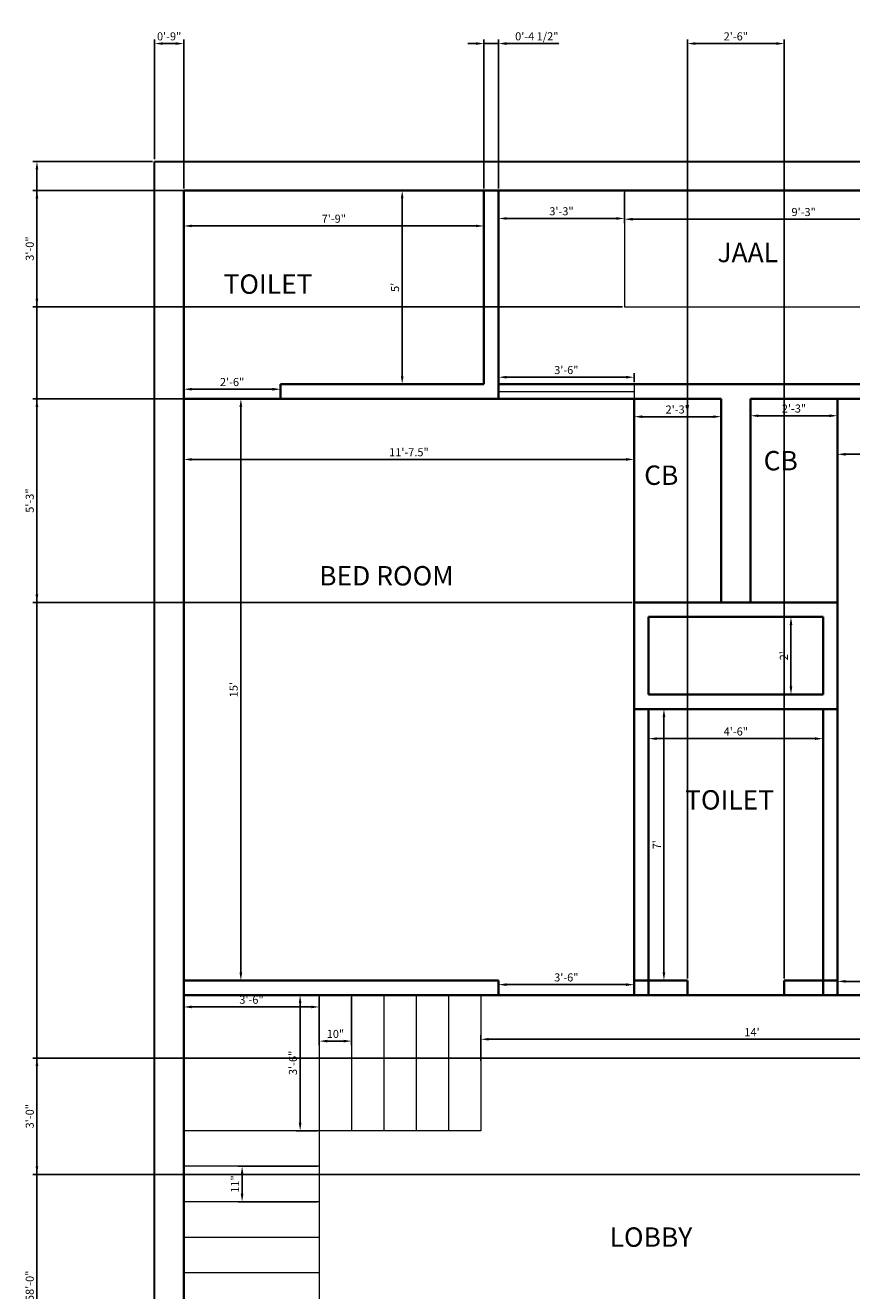
# Model space of a CAD drawing. Units: inches. Extents: x 2279 to 2719, y 394 to 1171.
# Tile 2 of 3: x 2281 to 2537, y 779 to 1171. Entities that reach past the tile are written whole.
import ezdxf

# ---------------------------------------------------------------- set-up
doc = ezdxf.new("R2010")
doc.units = ezdxf.units.IN
for name, color, linetype, lineweight in [('A-ANNO-DIMS', 2, 'Continuous', 13), ('A-ANNO-TEXT', 7, 'Continuous', 18), ('A-AREA-IDEN', 7, 'Continuous', 25), ('A-FLOR-OPEN', 4, 'Continuous', 18), ('A-FLOR-STRS', 3, 'Continuous', 20), ('A-GLAZ', 4, 'Continuous', 18), ('A-WALL', 7, 'Continuous', 35), ('C-PROP', 7, 'Continuous', 30)]:
    doc.layers.add(name, color=color, linetype=linetype, lineweight=lineweight)
doc.styles.get("Standard").update_dxf_attribs({"font": 'arial.ttf'})
doc.dimstyles.new('ISO-25', dxfattribs={"dimtxt": 2.5, "dimasz": 2.5, "dimexe": 1.25, "dimexo": 0.625, "dimtad": 1, "dimdec": 1, "dimlunit": 3, "dimtxsty": 'Standard', "dimcen": 2.5, "dimadec": 0, "dimazin": 0, "dimtfac": 1, "dimtdec": 1, "dimtmove": 0, "dimatfit": 3, "dimfxl": 1, "dimarcsym": 0})

# ---------------------------------------------------------------- blocks, each defined once
blk = doc.blocks.new('*D1')
at = {"layer": 'A-ANNO-DIMS', "color": 0, "lineweight": -2, "transparency": 16777216}
for p, q in [((2330.14, 1118.83), (2330.14, 1107.21)), ((2423.14, 1118.83), (2423.14, 1107.21)), ((2332.64, 1108.46), (2420.64, 1108.46))]:
    blk.add_line(p, q, dxfattribs=at)
at = {"layer": 'A-ANNO-DIMS', "color": 0, "transparency": 16777216}
for points in [[(2332.64, 1108.88), (2332.64, 1108.05), (2330.14, 1108.46)], [(2420.64, 1108.88), (2420.64, 1108.05), (2423.14, 1108.46)]]:
    blk.add_solid(points, dxfattribs=at)
at = {"layer": 'Defpoints', "color": 0, "transparency": 16777216}
for p in [(2330.14, 1119.45), (2423.14, 1119.45), (2423.14, 1108.46)]:
    blk.add_point(p, dxfattribs=at)
at = {"layer": 'A-ANNO-DIMS', "color": 0, "transparency": 16777216, "insert": (2376.64, 1110.37), "char_height": 2.5, "attachment_point": 5}
blk.add_mtext('7\'-9"', dxfattribs=at)
blk = doc.blocks.new('*D2')
at = {"layer": 'A-ANNO-DIMS', "color": 0, "lineweight": -2, "transparency": 16777216}
for p, q in [((2422.52, 1119.45), (2396.56, 1119.45)), ((2397.81, 1116.95), (2397.81, 1061.95)), ((2422.52, 1059.45), (2396.56, 1059.45))]:
    blk.add_line(p, q, dxfattribs=at)
at = {"layer": 'A-ANNO-DIMS', "color": 0, "transparency": 16777216}
for points in [[(2397.4, 1116.95), (2398.23, 1116.95), (2397.81, 1119.45)], [(2397.4, 1061.95), (2398.23, 1061.95), (2397.81, 1059.45)]]:
    blk.add_solid(points, dxfattribs=at)
at = {"layer": 'Defpoints', "color": 0, "transparency": 16777216}
for p in [(2423.14, 1119.45), (2397.81, 1059.45), (2423.14, 1059.45)]:
    blk.add_point(p, dxfattribs=at)
at = {"layer": 'A-ANNO-DIMS', "color": 0, "transparency": 16777216, "insert": (2395.92, 1089.45), "char_height": 2.5, "attachment_point": 5, "rotation": 90}
blk.add_mtext("5'", dxfattribs=at)
blk = doc.blocks.new('*D3')
at = {"layer": 'A-ANNO-DIMS', "color": 0, "lineweight": -2, "transparency": 16777216}
for p, q in [((2427.64, 1118.83), (2427.64, 1109.52)), ((2466.64, 1118.83), (2466.64, 1109.52)), ((2430.14, 1110.77), (2464.14, 1110.77))]:
    blk.add_line(p, q, dxfattribs=at)
at = {"layer": 'A-ANNO-DIMS', "color": 0, "transparency": 16777216}
for points in [[(2430.14, 1111.19), (2430.14, 1110.35), (2427.64, 1110.77)], [(2464.14, 1111.19), (2464.14, 1110.35), (2466.64, 1110.77)]]:
    blk.add_solid(points, dxfattribs=at)
at = {"layer": 'Defpoints', "color": 0, "transparency": 16777216}
for p in [(2427.64, 1119.45), (2466.64, 1119.45), (2466.64, 1110.77)]:
    blk.add_point(p, dxfattribs=at)
at = {"layer": 'A-ANNO-DIMS', "color": 0, "transparency": 16777216, "insert": (2447.14, 1112.67), "char_height": 2.5, "attachment_point": 5}
blk.add_mtext('3\'-3"', dxfattribs=at)
blk = doc.blocks.new('*D5')
at = {"layer": 'A-ANNO-DIMS', "color": 0, "lineweight": -2, "transparency": 16777216}
for p, q in [((2466.64, 1118.83), (2466.64, 1109.29)), ((2577.64, 1118.83), (2577.64, 1109.29)), ((2469.14, 1110.54), (2575.14, 1110.54))]:
    blk.add_line(p, q, dxfattribs=at)
at = {"layer": 'A-ANNO-DIMS', "color": 0, "transparency": 16777216}
for points in [[(2469.14, 1110.95), (2469.14, 1110.12), (2466.64, 1110.54)], [(2575.14, 1110.95), (2575.14, 1110.12), (2577.64, 1110.54)]]:
    blk.add_solid(points, dxfattribs=at)
at = {"layer": 'Defpoints', "color": 0, "transparency": 16777216}
for p in [(2466.64, 1119.45), (2577.64, 1119.45), (2577.64, 1110.54)]:
    blk.add_point(p, dxfattribs=at)
at = {"layer": 'A-ANNO-DIMS', "color": 0, "transparency": 16777216, "insert": (2522.14, 1112.44), "char_height": 2.5, "attachment_point": 5}
blk.add_mtext('9\'-3"', dxfattribs=at)
blk = doc.blocks.new('*D9')
at = {"layer": 'A-ANNO-DIMS', "color": 0, "lineweight": -2, "transparency": 16777216}
for p, q in [((2330.14, 1054.33), (2330.14, 1034.95)), ((2469.64, 1054.33), (2469.64, 1034.95)), ((2332.64, 1036.2), (2467.14, 1036.2))]:
    blk.add_line(p, q, dxfattribs=at)
at = {"layer": 'A-ANNO-DIMS', "color": 0, "transparency": 16777216}
for points in [[(2332.64, 1036.62), (2332.64, 1035.78), (2330.14, 1036.2)], [(2467.14, 1036.62), (2467.14, 1035.78), (2469.64, 1036.2)]]:
    blk.add_solid(points, dxfattribs=at)
at = {"layer": 'Defpoints', "color": 0, "transparency": 16777216}
for p in [(2330.14, 1054.95), (2469.64, 1054.95), (2469.64, 1036.2)]:
    blk.add_point(p, dxfattribs=at)
at = {"layer": 'A-ANNO-DIMS', "color": 0, "transparency": 16777216, "insert": (2399.89, 1038.1), "char_height": 2.5, "attachment_point": 5}
blk.add_mtext('11\'-7.5"', dxfattribs=at)
blk = doc.blocks.new('*D10')
at = {"layer": 'A-ANNO-DIMS', "color": 0, "lineweight": -2, "transparency": 16777216}
for p, q in [((2330.77, 1054.95), (2349.09, 1054.95)), ((2347.84, 1052.45), (2347.84, 877.45)), ((2330.77, 874.95), (2349.09, 874.95))]:
    blk.add_line(p, q, dxfattribs=at)
at = {"layer": 'A-ANNO-DIMS', "color": 0, "transparency": 16777216}
for points in [[(2347.42, 1052.45), (2348.26, 1052.45), (2347.84, 1054.95)], [(2347.42, 877.45), (2348.26, 877.45), (2347.84, 874.95)]]:
    blk.add_solid(points, dxfattribs=at)
at = {"layer": 'Defpoints', "color": 0, "transparency": 16777216}
for p in [(2330.14, 1054.95), (2330.14, 874.95), (2347.84, 874.95)]:
    blk.add_point(p, dxfattribs=at)
at = {"layer": 'A-ANNO-DIMS', "color": 0, "transparency": 16777216, "insert": (2345.94, 964.95), "char_height": 2.5, "attachment_point": 5, "rotation": 90}
blk.add_mtext("15'", dxfattribs=at)
blk = doc.blocks.new('*D11')
at = {"layer": 'A-ANNO-DIMS', "color": 0, "lineweight": -2, "transparency": 16777216}
for p, q in [((2469.64, 1054.33), (2469.64, 1048.18)), ((2496.64, 1054.33), (2496.64, 1048.18)), ((2472.14, 1049.43), (2494.14, 1049.43))]:
    blk.add_line(p, q, dxfattribs=at)
at = {"layer": 'A-ANNO-DIMS', "color": 0, "transparency": 16777216}
for points in [[(2472.14, 1049.84), (2472.14, 1049.01), (2469.64, 1049.43)], [(2494.14, 1049.84), (2494.14, 1049.01), (2496.64, 1049.43)]]:
    blk.add_solid(points, dxfattribs=at)
at = {"layer": 'Defpoints', "color": 0, "transparency": 16777216}
for p in [(2469.64, 1054.95), (2496.64, 1054.95), (2496.64, 1049.43)]:
    blk.add_point(p, dxfattribs=at)
at = {"layer": 'A-ANNO-DIMS', "color": 0, "transparency": 16777216, "insert": (2483.14, 1051.33), "char_height": 2.5, "attachment_point": 5}
blk.add_mtext('2\'-3"', dxfattribs=at)
blk = doc.blocks.new('*D12')
at = {"layer": 'A-ANNO-DIMS', "color": 0, "lineweight": -2, "transparency": 16777216}
for p, q in [((2505.64, 1054.33), (2505.64, 1048.47)), ((2532.64, 1054.33), (2532.64, 1048.47)), ((2508.14, 1049.72), (2530.14, 1049.72))]:
    blk.add_line(p, q, dxfattribs=at)
at = {"layer": 'A-ANNO-DIMS', "color": 0, "transparency": 16777216}
for points in [[(2508.14, 1050.13), (2508.14, 1049.3), (2505.64, 1049.72)], [(2530.14, 1050.13), (2530.14, 1049.3), (2532.64, 1049.72)]]:
    blk.add_solid(points, dxfattribs=at)
at = {"layer": 'Defpoints', "color": 0, "transparency": 16777216}
for p in [(2505.64, 1054.95), (2532.64, 1054.95), (2532.64, 1049.72)]:
    blk.add_point(p, dxfattribs=at)
at = {"layer": 'A-ANNO-DIMS', "color": 0, "transparency": 16777216, "insert": (2519.14, 1051.62), "char_height": 2.5, "attachment_point": 5}
blk.add_mtext('2\'-3"', dxfattribs=at)
blk = doc.blocks.new('*D13')
at = {"layer": 'A-ANNO-DIMS', "color": 0, "lineweight": -2, "transparency": 16777216}
for p, q in [((2527.52, 987.45), (2516.96, 987.45)), ((2518.21, 984.95), (2518.21, 965.95)), ((2527.52, 963.45), (2516.96, 963.45))]:
    blk.add_line(p, q, dxfattribs=at)
at = {"layer": 'A-ANNO-DIMS', "color": 0, "transparency": 16777216}
for points in [[(2517.8, 984.95), (2518.63, 984.95), (2518.21, 987.45)], [(2517.8, 965.95), (2518.63, 965.95), (2518.21, 963.45)]]:
    blk.add_solid(points, dxfattribs=at)
at = {"layer": 'Defpoints', "color": 0, "transparency": 16777216}
for p in [(2528.14, 987.45), (2518.21, 963.45), (2528.14, 963.45)]:
    blk.add_point(p, dxfattribs=at)
at = {"layer": 'A-ANNO-DIMS', "color": 0, "transparency": 16777216, "insert": (2516.33, 975.45), "char_height": 2.5, "attachment_point": 5, "rotation": 90}
blk.add_mtext("2'", dxfattribs=at)
blk = doc.blocks.new('*D14')
at = {"layer": 'A-ANNO-DIMS', "color": 0, "lineweight": -2, "transparency": 16777216}
for p, q in [((2474.77, 958.95), (2480.12, 958.95)), ((2478.87, 956.45), (2478.87, 877.45)), ((2474.77, 874.95), (2480.12, 874.95))]:
    blk.add_line(p, q, dxfattribs=at)
at = {"layer": 'A-ANNO-DIMS', "color": 0, "transparency": 16777216}
for points in [[(2478.45, 956.45), (2479.29, 956.45), (2478.87, 958.95)], [(2478.45, 877.45), (2479.29, 877.45), (2478.87, 874.95)]]:
    blk.add_solid(points, dxfattribs=at)
at = {"layer": 'Defpoints', "color": 0, "transparency": 16777216}
for p in [(2474.14, 958.95), (2474.14, 874.95), (2478.87, 874.95)]:
    blk.add_point(p, dxfattribs=at)
at = {"layer": 'A-ANNO-DIMS', "color": 0, "transparency": 16777216, "insert": (2477, 916.95), "char_height": 2.5, "attachment_point": 5, "rotation": 90}
blk.add_mtext("7'", dxfattribs=at)
blk = doc.blocks.new('*D15')
at = {"layer": 'A-ANNO-DIMS', "color": 0, "lineweight": -2, "transparency": 16777216}
for p, q in [((2474.14, 958.33), (2474.14, 948.54)), ((2528.14, 958.33), (2528.14, 948.54)), ((2476.64, 949.79), (2525.64, 949.79))]:
    blk.add_line(p, q, dxfattribs=at)
at = {"layer": 'A-ANNO-DIMS', "color": 0, "transparency": 16777216}
for points in [[(2476.64, 950.21), (2476.64, 949.37), (2474.14, 949.79)], [(2525.64, 950.21), (2525.64, 949.37), (2528.14, 949.79)]]:
    blk.add_solid(points, dxfattribs=at)
at = {"layer": 'Defpoints', "color": 0, "transparency": 16777216}
for p in [(2474.14, 958.95), (2528.14, 958.95), (2528.14, 949.79)]:
    blk.add_point(p, dxfattribs=at)
at = {"layer": 'A-ANNO-DIMS', "color": 0, "transparency": 16777216, "insert": (2501.14, 951.69), "char_height": 2.5, "attachment_point": 5}
blk.add_mtext('4\'-6"', dxfattribs=at)
blk = doc.blocks.new('*D16')
at = {"layer": 'A-ANNO-DIMS', "color": 0, "lineweight": -2, "transparency": 16777216}
for p, q in [((2532.64, 1054.33), (2532.64, 1036.54)), ((2672.14, 1054.33), (2672.14, 1036.54)), ((2535.14, 1037.79), (2669.64, 1037.79))]:
    blk.add_line(p, q, dxfattribs=at)
at = {"layer": 'A-ANNO-DIMS', "color": 0, "transparency": 16777216}
for points in [[(2535.14, 1038.21), (2535.14, 1037.37), (2532.64, 1037.79)], [(2669.64, 1038.21), (2669.64, 1037.37), (2672.14, 1037.79)]]:
    blk.add_solid(points, dxfattribs=at)
at = {"layer": 'Defpoints', "color": 0, "transparency": 16777216}
for p in [(2532.64, 1054.95), (2672.14, 1054.95), (2672.14, 1037.79)]:
    blk.add_point(p, dxfattribs=at)
at = {"layer": 'A-ANNO-DIMS', "color": 0, "transparency": 16777216, "insert": (2602.39, 1039.69), "char_height": 2.5, "attachment_point": 5}
blk.add_mtext('11\'-7.5"', dxfattribs=at)
blk = doc.blocks.new('*D18')
at = {"layer": 'A-ANNO-DIMS', "color": 0, "lineweight": -2, "transparency": 16777216}
for p, q in [((2330.14, 869.83), (2330.14, 865.51)), ((2372.14, 869.83), (2372.14, 865.51)), ((2332.64, 866.76), (2369.64, 866.76))]:
    blk.add_line(p, q, dxfattribs=at)
at = {"layer": 'A-ANNO-DIMS', "color": 0, "transparency": 16777216}
for points in [[(2332.64, 867.18), (2332.64, 866.35), (2330.14, 866.76)], [(2369.64, 867.18), (2369.64, 866.35), (2372.14, 866.76)]]:
    blk.add_solid(points, dxfattribs=at)
at = {"layer": 'Defpoints', "color": 0, "transparency": 16777216}
for p in [(2330.14, 870.45), (2372.14, 870.45), (2372.14, 866.76)]:
    blk.add_point(p, dxfattribs=at)
at = {"layer": 'A-ANNO-DIMS', "color": 0, "transparency": 16777216, "insert": (2351.14, 868.67), "char_height": 2.5, "attachment_point": 5}
blk.add_mtext('3\'-6"', dxfattribs=at)
blk = doc.blocks.new('*D19')
at = {"layer": 'A-ANNO-DIMS', "color": 0, "lineweight": -2, "transparency": 16777216}
for p, q in [((2371.52, 870.45), (2364.95, 870.45)), ((2366.2, 830.95), (2366.2, 867.95)), ((2371.52, 828.45), (2364.95, 828.45))]:
    blk.add_line(p, q, dxfattribs=at)
at = {"layer": 'A-ANNO-DIMS', "color": 0, "transparency": 16777216}
for points in [[(2365.79, 867.95), (2366.62, 867.95), (2366.2, 870.45)], [(2365.79, 830.95), (2366.62, 830.95), (2366.2, 828.45)]]:
    blk.add_solid(points, dxfattribs=at)
at = {"layer": 'Defpoints', "color": 0, "transparency": 16777216}
for p in [(2366.2, 870.45), (2372.14, 870.45), (2372.14, 828.45)]:
    blk.add_point(p, dxfattribs=at)
at = {"layer": 'A-ANNO-DIMS', "color": 0, "transparency": 16777216, "insert": (2364.3, 849.45), "char_height": 2.5, "attachment_point": 5, "rotation": 90}
blk.add_mtext('3\'-6"', dxfattribs=at)
blk = doc.blocks.new('*D20')
at = {"layer": 'A-ANNO-DIMS', "color": 0, "lineweight": -2, "transparency": 16777216}
for p, q in [((2372.14, 869.83), (2372.14, 854.94)), ((2382.14, 869.83), (2382.14, 854.94)), ((2374.64, 856.19), (2379.64, 856.19))]:
    blk.add_line(p, q, dxfattribs=at)
at = {"layer": 'A-ANNO-DIMS', "color": 0, "transparency": 16777216}
for points in [[(2374.64, 856.61), (2374.64, 855.77), (2372.14, 856.19)], [(2379.64, 856.61), (2379.64, 855.77), (2382.14, 856.19)]]:
    blk.add_solid(points, dxfattribs=at)
at = {"layer": 'Defpoints', "color": 0, "transparency": 16777216}
for p in [(2372.14, 870.45), (2382.14, 870.45), (2382.14, 856.19)]:
    blk.add_point(p, dxfattribs=at)
at = {"layer": 'A-ANNO-DIMS', "color": 0, "transparency": 16777216, "insert": (2377.14, 858.09), "char_height": 2.5, "attachment_point": 5}
blk.add_mtext('10"', dxfattribs=at)
blk = doc.blocks.new('*D21')
at = {"layer": 'A-ANNO-DIMS', "color": 0, "lineweight": -2, "transparency": 16777216}
for p, q in [((2371.52, 817.45), (2346.98, 817.45)), ((2348.23, 814.95), (2348.23, 808.95)), ((2371.52, 806.45), (2346.98, 806.45))]:
    blk.add_line(p, q, dxfattribs=at)
at = {"layer": 'A-ANNO-DIMS', "color": 0, "transparency": 16777216}
for points in [[(2347.81, 814.95), (2348.64, 814.95), (2348.23, 817.45)], [(2347.81, 808.95), (2348.64, 808.95), (2348.23, 806.45)]]:
    blk.add_solid(points, dxfattribs=at)
at = {"layer": 'Defpoints', "color": 0, "transparency": 16777216}
for p in [(2372.14, 817.45), (2348.23, 806.45), (2372.14, 806.45)]:
    blk.add_point(p, dxfattribs=at)
at = {"layer": 'A-ANNO-DIMS', "color": 0, "transparency": 16777216, "insert": (2346.35, 811.95), "char_height": 2.5, "attachment_point": 5, "rotation": 90}
blk.add_mtext('11"', dxfattribs=at)
blk = doc.blocks.new('*D34')
at = {"layer": 'A-ANNO-DIMS', "color": 0, "lineweight": -2, "transparency": 16777216}
for p, q in [((2422.14, 850.08), (2422.14, 858.01)), ((2590.14, 850.08), (2590.14, 858.01)), ((2424.64, 856.76), (2587.64, 856.76))]:
    blk.add_line(p, q, dxfattribs=at)
at = {"layer": 'A-ANNO-DIMS', "color": 0, "transparency": 16777216}
for points in [[(2424.64, 857.18), (2424.64, 856.35), (2422.14, 856.76)], [(2587.64, 857.18), (2587.64, 856.35), (2590.14, 856.76)]]:
    blk.add_solid(points, dxfattribs=at)
at = {"layer": 'Defpoints', "color": 0, "transparency": 16777216}
for p in [(2590.14, 856.76), (2422.14, 849.45), (2590.14, 849.45)]:
    blk.add_point(p, dxfattribs=at)
at = {"layer": 'A-ANNO-DIMS', "color": 0, "transparency": 16777216, "insert": (2506.14, 858.64), "char_height": 2.5, "attachment_point": 5}
blk.add_mtext("14'", dxfattribs=at)
blk = doc.blocks.new('*U37')
for p, q in [((0, 100), (0, 0)), ((900, 100), (900, 0)), ((0, 50), (900, 50))]:
    blk.add_line(p, q)
blk = doc.blocks.new('*D39')
at = {"layer": 'A-ANNO-DIMS', "color": 0, "lineweight": -2, "transparency": 16777216}
for p, q in [((2330.14, 1058.83), (2330.14, 1056.68)), ((2357.64, 1057.93), (2332.64, 1057.93)), ((2360.14, 1058.83), (2360.14, 1056.68))]:
    blk.add_line(p, q, dxfattribs=at)
at = {"layer": 'A-ANNO-DIMS', "color": 0, "transparency": 16777216}
for points in [[(2332.64, 1058.34), (2332.64, 1057.51), (2330.14, 1057.93)], [(2357.64, 1058.34), (2357.64, 1057.51), (2360.14, 1057.93)]]:
    blk.add_solid(points, dxfattribs=at)
at = {"layer": 'Defpoints', "color": 0, "transparency": 16777216}
for p in [(2330.14, 1059.45), (2330.14, 1057.93), (2360.14, 1059.45)]:
    blk.add_point(p, dxfattribs=at)
at = {"layer": 'A-ANNO-DIMS', "color": 0, "transparency": 16777216, "insert": (2345.14, 1059.83), "char_height": 2.5, "attachment_point": 5}
blk.add_mtext('2\'-6"', dxfattribs=at)
blk = doc.blocks.new('*D40')
at = {"layer": 'A-ANNO-DIMS', "color": 0, "lineweight": -2, "transparency": 16777216}
for p, q in [((2427.64, 1060.08), (2427.64, 1062.89)), ((2430.14, 1061.64), (2467.14, 1061.64)), ((2469.64, 1060.08), (2469.64, 1062.89))]:
    blk.add_line(p, q, dxfattribs=at)
at = {"layer": 'A-ANNO-DIMS', "color": 0, "transparency": 16777216}
for points in [[(2430.14, 1062.06), (2430.14, 1061.23), (2427.64, 1061.64)], [(2467.14, 1062.06), (2467.14, 1061.23), (2469.64, 1061.64)]]:
    blk.add_solid(points, dxfattribs=at)
at = {"layer": 'Defpoints', "color": 0, "transparency": 16777216}
for p in [(2469.64, 1061.64), (2427.64, 1059.45), (2469.64, 1059.45)]:
    blk.add_point(p, dxfattribs=at)
at = {"layer": 'A-ANNO-DIMS', "color": 0, "transparency": 16777216, "insert": (2448.64, 1063.54), "char_height": 2.5, "attachment_point": 5}
blk.add_mtext('3\'-6"', dxfattribs=at)
blk = doc.blocks.new('*D42')
at = {"layer": 'A-ANNO-DIMS', "color": 0, "lineweight": -2, "transparency": 16777216}
for p, q in [((2427.64, 871.08), (2427.64, 874.92)), ((2430.14, 873.67), (2467.14, 873.67)), ((2469.64, 871.08), (2469.64, 874.92))]:
    blk.add_line(p, q, dxfattribs=at)
at = {"layer": 'A-ANNO-DIMS', "color": 0, "transparency": 16777216}
for points in [[(2430.14, 874.08), (2430.14, 873.25), (2427.64, 873.67)], [(2467.14, 874.08), (2467.14, 873.25), (2469.64, 873.67)]]:
    blk.add_solid(points, dxfattribs=at)
at = {"layer": 'Defpoints', "color": 0, "transparency": 16777216}
for p in [(2469.64, 873.67), (2427.64, 870.45), (2469.64, 870.45)]:
    blk.add_point(p, dxfattribs=at)
at = {"layer": 'A-ANNO-DIMS', "color": 0, "transparency": 16777216, "insert": (2448.64, 875.57), "char_height": 2.5, "attachment_point": 5}
blk.add_mtext('3\'-6"', dxfattribs=at)
blk = doc.blocks.new('*D43')
at = {"layer": 'A-ANNO-DIMS', "color": 0, "lineweight": -2, "transparency": 16777216}
for p, q in [((2532.64, 871.08), (2532.64, 875.93)), ((2572.14, 874.68), (2535.14, 874.68)), ((2574.64, 871.08), (2574.64, 875.93))]:
    blk.add_line(p, q, dxfattribs=at)
at = {"layer": 'A-ANNO-DIMS', "color": 0, "transparency": 16777216}
for points in [[(2535.14, 875.1), (2535.14, 874.26), (2532.64, 874.68)], [(2572.14, 875.1), (2572.14, 874.26), (2574.64, 874.68)]]:
    blk.add_solid(points, dxfattribs=at)
at = {"layer": 'Defpoints', "color": 0, "transparency": 16777216}
for p in [(2532.64, 874.68), (2532.64, 870.45), (2574.64, 870.45)]:
    blk.add_point(p, dxfattribs=at)
at = {"layer": 'A-ANNO-DIMS', "color": 0, "transparency": 16777216, "insert": (2553.64, 876.58), "char_height": 2.5, "attachment_point": 5}
blk.add_mtext('3\'-6"', dxfattribs=at)
blk = doc.blocks.new('*D57')
at = {"layer": 'A-ANNO-DIMS', "color": 0, "lineweight": -2, "transparency": 16777216}
for p, q in [((2321.14, 1129.08), (2321.14, 1166.15)), ((2323.64, 1164.9), (2327.64, 1164.9)), ((2330.14, 1120.08), (2330.14, 1166.15))]:
    blk.add_line(p, q, dxfattribs=at)
at = {"layer": 'A-ANNO-DIMS', "color": 0, "transparency": 16777216}
for points in [[(2323.64, 1165.32), (2323.64, 1164.48), (2321.14, 1164.9)], [(2327.64, 1165.32), (2327.64, 1164.48), (2330.14, 1164.9)]]:
    blk.add_solid(points, dxfattribs=at)
at = {"layer": 'Defpoints', "color": 0, "transparency": 16777216}
for p in [(2330.14, 1164.9), (2321.14, 1128.45), (2330.14, 1119.45)]:
    blk.add_point(p, dxfattribs=at)
at = {"layer": 'A-ANNO-DIMS', "color": 0, "transparency": 16777216, "insert": (2325.64, 1166.8), "char_height": 2.5, "attachment_point": 5}
blk.add_mtext('0\'-9"', dxfattribs=at)
blk = doc.blocks.new('*D58')
at = {"layer": 'A-ANNO-DIMS', "color": 0, "lineweight": -2, "transparency": 16777216}
for p, q in [((2420.64, 1164.9), (2418.14, 1164.9)), ((2423.14, 1120.08), (2423.14, 1166.15)), ((2423.14, 1164.9), (2427.64, 1164.9)), ((2427.64, 1120.08), (2427.64, 1166.15)), ((2430.14, 1164.9), (2446.36, 1164.9))]:
    blk.add_line(p, q, dxfattribs=at)
at = {"layer": 'A-ANNO-DIMS', "color": 0, "transparency": 16777216}
for points in [[(2420.64, 1165.32), (2420.64, 1164.48), (2423.14, 1164.9)], [(2430.14, 1165.32), (2430.14, 1164.48), (2427.64, 1164.9)]]:
    blk.add_solid(points, dxfattribs=at)
at = {"layer": 'Defpoints', "color": 0, "transparency": 16777216}
for p in [(2427.64, 1164.9), (2423.14, 1119.45), (2427.64, 1119.45)]:
    blk.add_point(p, dxfattribs=at)
at = {"layer": 'A-ANNO-DIMS', "color": 0, "transparency": 16777216, "insert": (2439.5, 1166.82), "char_height": 2.5, "attachment_point": 5}
blk.add_mtext('0\'-4 1/2"', dxfattribs=at)
blk = doc.blocks.new('*D59')
at = {"layer": 'A-ANNO-DIMS', "color": 0, "lineweight": -2, "transparency": 16777216}
for p, q in [((2466.02, 1119.45), (2283.44, 1119.45)), ((2284.69, 1116.95), (2284.69, 1085.95)), ((2466.02, 1083.45), (2283.44, 1083.45))]:
    blk.add_line(p, q, dxfattribs=at)
at = {"layer": 'A-ANNO-DIMS', "color": 0, "transparency": 16777216}
for points in [[(2284.27, 1116.95), (2285.11, 1116.95), (2284.69, 1119.45)], [(2284.27, 1085.95), (2285.11, 1085.95), (2284.69, 1083.45)]]:
    blk.add_solid(points, dxfattribs=at)
at = {"layer": 'Defpoints', "color": 0, "transparency": 16777216}
for p in [(2466.64, 1119.45), (2284.69, 1083.45), (2466.64, 1083.45)]:
    blk.add_point(p, dxfattribs=at)
at = {"layer": 'A-ANNO-DIMS', "color": 0, "transparency": 16777216, "insert": (2282.79, 1101.45), "char_height": 2.5, "attachment_point": 5, "rotation": 90}
blk.add_mtext('3\'-0"', dxfattribs=at)
blk = doc.blocks.new('*D61')
at = {"layer": 'A-ANNO-DIMS', "color": 0, "lineweight": -2, "transparency": 16777216}
for p, q in [((2486.14, 875.58), (2486.14, 1166.15)), ((2488.64, 1164.9), (2513.64, 1164.9)), ((2516.14, 875.58), (2516.14, 1166.15))]:
    blk.add_line(p, q, dxfattribs=at)
at = {"layer": 'A-ANNO-DIMS', "color": 0, "transparency": 16777216}
for points in [[(2488.64, 1165.32), (2488.64, 1164.48), (2486.14, 1164.9)], [(2513.64, 1165.32), (2513.64, 1164.48), (2516.14, 1164.9)]]:
    blk.add_solid(points, dxfattribs=at)
at = {"layer": 'Defpoints', "color": 0, "transparency": 16777216}
for p in [(2516.14, 1164.9), (2486.14, 874.95), (2516.14, 874.95)]:
    blk.add_point(p, dxfattribs=at)
at = {"layer": 'A-ANNO-DIMS', "color": 0, "transparency": 16777216, "insert": (2501.14, 1166.8), "char_height": 2.5, "attachment_point": 5}
blk.add_mtext('2\'-6"', dxfattribs=at)
blk = doc.blocks.new('*D62')
at = {"layer": 'A-ANNO-DIMS', "color": 0, "lineweight": -2, "transparency": 16777216}
for p, q in [((2594.02, 850.95), (2283.44, 850.95)), ((2284.69, 848.45), (2284.69, 817.45)), ((2589.52, 814.95), (2283.44, 814.95))]:
    blk.add_line(p, q, dxfattribs=at)
at = {"layer": 'A-ANNO-DIMS', "color": 0, "transparency": 16777216}
for points in [[(2284.27, 848.45), (2285.11, 848.45), (2284.69, 850.95)], [(2284.27, 817.45), (2285.11, 817.45), (2284.69, 814.95)]]:
    blk.add_solid(points, dxfattribs=at)
at = {"layer": 'Defpoints', "color": 0, "transparency": 16777216}
for p in [(2594.64, 850.95), (2284.69, 814.95), (2590.14, 814.95)]:
    blk.add_point(p, dxfattribs=at)
at = {"layer": 'A-ANNO-DIMS', "color": 0, "transparency": 16777216, "insert": (2282.79, 832.95), "char_height": 2.5, "attachment_point": 5, "rotation": 90}
blk.add_mtext('3\'-0"', dxfattribs=at)
blk = doc.blocks.new('*D66')
at = {"layer": 'A-ANNO-DIMS', "color": 0, "lineweight": -2, "transparency": 16777216}
for p, q in [((2469.02, 1054.95), (2283.44, 1054.95)), ((2284.69, 994.45), (2284.69, 1052.45)), ((2469.02, 991.95), (2283.44, 991.95))]:
    blk.add_line(p, q, dxfattribs=at)
at = {"layer": 'A-ANNO-DIMS', "color": 0, "transparency": 16777216}
for points in [[(2284.27, 1052.45), (2285.11, 1052.45), (2284.69, 1054.95)], [(2284.27, 994.45), (2285.11, 994.45), (2284.69, 991.95)]]:
    blk.add_solid(points, dxfattribs=at)
at = {"layer": 'Defpoints', "color": 0, "transparency": 16777216}
for p in [(2284.69, 1054.95), (2469.64, 1054.95), (2469.64, 991.95)]:
    blk.add_point(p, dxfattribs=at)
at = {"layer": 'A-ANNO-DIMS', "color": 0, "transparency": 16777216, "insert": (2282.79, 1023.45), "char_height": 2.5, "attachment_point": 5, "rotation": 90}
blk.add_mtext('5\'-3"', dxfattribs=at)
blk = doc.blocks.new('*D68')
at = {"layer": 'A-ANNO-DIMS', "color": 0, "lineweight": -2, "transparency": 16777216}
for p, q in [((2320.52, 1128.45), (2283.44, 1128.45)), ((2284.69, 434.95), (2284.69, 1125.95)), ((2320.52, 432.45), (2283.44, 432.45))]:
    blk.add_line(p, q, dxfattribs=at)
at = {"layer": 'A-ANNO-DIMS', "color": 0, "transparency": 16777216}
for points in [[(2284.27, 1125.95), (2285.11, 1125.95), (2284.69, 1128.45)], [(2284.27, 434.95), (2285.11, 434.95), (2284.69, 432.45)]]:
    blk.add_solid(points, dxfattribs=at)
at = {"layer": 'Defpoints', "color": 0, "transparency": 16777216}
for p in [(2284.69, 1128.45), (2321.14, 1128.45), (2321.14, 432.45)]:
    blk.add_point(p, dxfattribs=at)
at = {"layer": 'A-ANNO-DIMS', "color": 0, "transparency": 16777216, "insert": (2282.79, 780.45), "char_height": 2.5, "attachment_point": 5, "rotation": 90}
blk.add_mtext('58\'-0"', dxfattribs=at)

msp = doc.modelspace()

# ---------------------------------------------------------------- linework, layer by layer
at = {"layer": 'A-FLOR-OPEN'}
for p, q in [((2466.64, 1119.45), (2466.64, 1083.45)), ((2466.64, 1083.45), (2577.64, 1083.45))]:
    msp.add_line(p, q, dxfattribs=at)
at = {"layer": 'A-FLOR-STRS'}
for p, q in [((2372.14, 870.45), (2372.14, 709.95)), ((2382.14, 870.45), (2382.14, 828.45)), ((2382.14, 870.45), (2382.14, 828.45)), ((2392.14, 870.45), (2392.14, 828.45)), ((2402.14, 870.45), (2402.14, 828.45)), ((2412.14, 870.45), (2412.14, 828.45)), ((2422.14, 870.45), (2422.14, 828.45)), ((2372.14, 828.45), (2330.14, 828.45)), ((2422.14, 828.45), (2372.14, 828.45)), ((2372.14, 817.45), (2330.14, 817.45)), ((2372.14, 806.45), (2330.14, 806.45)), ((2372.14, 795.45), (2330.14, 795.45)), ((2372.14, 784.45), (2330.14, 784.45))]:
    msp.add_line(p, q, dxfattribs=at)
at = {"layer": 'A-GLAZ'}
msp.add_line((2469.64, 1059.45), (2469.64, 1054.95), dxfattribs=at)
at = {"layer": 'A-WALL'}
for p, q in [((2330.14, 1119.45), (2672.14, 1119.45)), ((2330.14, 552.45), (2330.14, 1119.45)), ((2423.14, 1059.45), (2423.14, 1119.45)), ((2427.64, 1054.95), (2427.64, 1119.45)), ((2360.14, 1059.45), (2423.14, 1059.45)), ((2360.14, 1059.45), (2360.14, 1054.95)), ((2427.64, 1059.45), (2621.14, 1059.45)), ((2330.14, 1054.95), (2496.64, 1054.95)), ((2469.64, 870.45), (2469.64, 1054.95)), ((2496.64, 991.95), (2496.64, 1054.95)), ((2505.64, 1054.95), (2505.64, 991.95)), ((2505.64, 1054.95), (2672.14, 1054.95)), ((2532.64, 1054.95), (2532.64, 870.45)), ((2469.64, 991.95), (2532.64, 991.95)), ((2474.14, 987.45), (2528.14, 987.45)), ((2474.14, 963.45), (2474.14, 987.45)), ((2528.14, 987.45), (2528.14, 963.45)), ((2528.14, 963.45), (2474.14, 963.45)), ((2469.64, 958.95), (2532.64, 958.95)), ((2474.14, 870.45), (2474.14, 958.95)), ((2528.14, 958.95), (2528.14, 870.45)), ((2330.14, 874.95), (2427.64, 874.95)), ((2427.64, 874.95), (2427.64, 870.45)), ((2469.64, 874.95), (2486.14, 874.95)), ((2486.14, 874.95), (2486.14, 870.45)), ((2516.14, 870.45), (2516.14, 874.95)), ((2516.14, 874.95), (2532.64, 874.95)), ((2330.14, 870.45), (2469.64, 870.45)), ((2469.64, 870.45), (2672.14, 870.45))]:
    msp.add_line(p, q, dxfattribs=at)
at = {"layer": 'C-PROP'}
for p, q in [((2321.14, 1128.45), (2681.14, 1128.45)), ((2321.14, 552.45), (2321.14, 1128.45))]:
    msp.add_line(p, q, dxfattribs=at)

# ---------------------------------------------------------------- block references
at = {"layer": 'A-GLAZ', "xscale": 0.0466666666666665, "yscale": 0.0466666666666665, "zscale": 0.0466666666666665}
msp.add_blockref('*U37', (2427.64, 1054.87), dxfattribs=at)

# ---------------------------------------------------------------- texts
at = {"layer": 'A-ANNO-TEXT'}
for p in [(2509.74, 1032.81), (2472.75, 1028.32)]:
    msp.add_text('CB', height=6, dxfattribs=at).set_placement(p)
at = {"layer": 'A-AREA-IDEN'}
for s, p in [('JAAL', (2495.44, 1097.24)), ('TOILET', (2342.49, 1087.46)), ('BED ROOM', (2372.1, 997.2)), ('TOILET', (2485.42, 927.84)), ('LOBBY', (2462.04, 792.54))]:
    msp.add_text(s, height=6, dxfattribs=at).set_placement(p)

# ---------------------------------------------------------------- dimensions: what is measured, and where the dimension line sits
at = {"layer": 'A-ANNO-DIMS'}
for base, p1, p2, override, picture, middle in [((2330.14, 1164.9), (2321.14, 1128.45), (2330.14, 1119.45), {"dimdec": 1, "dimlfac": 1, "dimrnd": 0, "dimzin": 1, "dimdsep": 46, "dimlunit": 4, "dimfrac": 2}, '*D57', (2325.64, 1166.8)), ((2427.64, 1164.9), (2423.14, 1119.45), (2427.64, 1119.45), {"dimdec": 1, "dimlfac": 1, "dimrnd": 0, "dimzin": 1, "dimdsep": 46, "dimlunit": 4, "dimfrac": 2}, '*D58', (2439.5, 1166.82)), ((2516.14, 1164.9), (2486.14, 874.95), (2516.14, 874.95), {"dimdec": 1, "dimlfac": 1, "dimrnd": 0, "dimzin": 1, "dimdsep": 46, "dimlunit": 4, "dimfrac": 2}, '*D61', (2501.14, 1166.8)), ((2423.14, 1108.46), (2330.14, 1119.45), (2423.14, 1119.45), {"dimclrd": 0, "dimclre": 0, "dimclrt": 0}, '*D1', (2376.64, 1110.37)), ((2466.64, 1110.77), (2427.64, 1119.45), (2466.64, 1119.45), {"dimclrd": 0, "dimclre": 0, "dimclrt": 0}, '*D3', (2447.14, 1112.67)), ((2577.64, 1110.54), (2466.64, 1119.45), (2577.64, 1119.45), {"dimclrd": 0, "dimclre": 0, "dimclrt": 0}, '*D5', (2522.14, 1112.44)), ((2469.64, 1061.64), (2427.64, 1059.45), (2469.64, 1059.45), {"dimclrd": 0, "dimclre": 0, "dimclrt": 0}, '*D40', (2448.64, 1063.54)), ((2330.14, 1057.93), (2360.14, 1059.45), (2330.14, 1059.45), {"dimclrd": 0, "dimclre": 0, "dimclrt": 0}, '*D39', (2345.14, 1059.83)), ((2469.64, 1036.2), (2330.14, 1054.95), (2469.64, 1054.95), {"dimclrd": 0, "dimclre": 0, "dimclrt": 0}, '*D9', (2399.89, 1038.1)), ((2496.64, 1049.43), (2469.64, 1054.95), (2496.64, 1054.95), {"dimclrd": 0, "dimclre": 0, "dimclrt": 0}, '*D11', (2483.14, 1051.33)), ((2532.64, 1049.72), (2505.64, 1054.95), (2532.64, 1054.95), {"dimclrd": 0, "dimclre": 0, "dimclrt": 0}, '*D12', (2519.14, 1051.62)), ((2672.14, 1037.79), (2532.64, 1054.95), (2672.14, 1054.95), {"dimclrd": 0, "dimclre": 0, "dimclrt": 0}, '*D16', (2602.39, 1039.69)), ((2528.14, 949.79), (2474.14, 958.95), (2528.14, 958.95), {"dimclrd": 0, "dimclre": 0, "dimclrt": 0}, '*D15', (2501.14, 951.69)), ((2469.64, 873.67), (2427.64, 870.45), (2469.64, 870.45), {"dimclrd": 0, "dimclre": 0, "dimclrt": 0}, '*D42', (2448.64, 875.57)), ((2532.64, 874.68), (2574.64, 870.45), (2532.64, 870.45), {"dimclrd": 0, "dimclre": 0, "dimclrt": 0}, '*D43', (2553.64, 876.58)), ((2372.14, 866.76), (2330.14, 870.45), (2372.14, 870.45), {"dimclrd": 0, "dimclre": 0, "dimclrt": 0}, '*D18', (2351.14, 868.67)), ((2382.14, 856.19), (2372.14, 870.45), (2382.14, 870.45), {"dimclrd": 0, "dimclre": 0, "dimclrt": 0}, '*D20', (2377.14, 858.09)), ((2590.14, 856.76), (2422.14, 849.45), (2590.14, 849.45), {"dimclrd": 0, "dimclre": 0, "dimclrt": 0}, '*D34', (2506.14, 858.64))]:
    dim = msp.add_linear_dim(base=base, p1=p1, p2=p2, dimstyle='ISO-25', override=override, dxfattribs=at)
    dim.commit()
    dim.dimension.update_dxf_attribs({"geometry": picture, "text_midpoint": middle})
for base, p1, p2, override, picture, middle in [((2284.69, 1128.45), (2321.14, 432.45), (2321.14, 1128.45), {"dimdec": 1, "dimlfac": 1, "dimrnd": 0, "dimzin": 1, "dimdsep": 46, "dimlunit": 4, "dimfrac": 2}, '*D68', (2282.79, 780.45)), ((2284.69, 1083.45), (2466.64, 1119.45), (2466.64, 1083.45), {"dimdec": 1, "dimlfac": 1, "dimrnd": 0, "dimzin": 1, "dimdsep": 46, "dimlunit": 4, "dimfrac": 2}, '*D59', (2282.79, 1101.45)), ((2397.81, 1059.45), (2423.14, 1119.45), (2423.14, 1059.45), {"dimclrd": 0, "dimclre": 0, "dimclrt": 0}, '*D2', (2395.92, 1089.45)), ((2284.69, 1054.95), (2469.64, 991.95), (2469.64, 1054.95), {"dimdec": 1, "dimlfac": 1, "dimrnd": 0, "dimzin": 1, "dimdsep": 46, "dimlunit": 4, "dimfrac": 2}, '*D66', (2282.79, 1023.45)), ((2347.84, 874.95), (2330.14, 1054.95), (2330.14, 874.95), {"dimclrd": 0, "dimclre": 0, "dimclrt": 0}, '*D10', (2345.94, 964.95)), ((2518.21, 963.45), (2528.14, 987.45), (2528.14, 963.45), {"dimclrd": 0, "dimclre": 0, "dimclrt": 0}, '*D13', (2516.33, 975.45)), ((2478.87, 874.95), (2474.14, 958.95), (2474.14, 874.95), {"dimclrd": 0, "dimclre": 0, "dimclrt": 0}, '*D14', (2477, 916.95)), ((2366.2, 870.45), (2372.14, 828.45), (2372.14, 870.45), {"dimclrd": 0, "dimclre": 0, "dimclrt": 0}, '*D19', (2364.3, 849.45)), ((2284.69, 814.95), (2594.64, 850.95), (2590.14, 814.95), {"dimdec": 1, "dimlfac": 1, "dimrnd": 0, "dimzin": 1, "dimdsep": 46, "dimlunit": 4, "dimfrac": 2}, '*D62', (2282.79, 832.95)), ((2348.23, 806.45), (2372.14, 817.45), (2372.14, 806.45), {"dimclrd": 0, "dimclre": 0, "dimclrt": 0}, '*D21', (2346.35, 811.95))]:
    dim = msp.add_linear_dim(base=base, p1=p1, p2=p2, angle=90, dimstyle='ISO-25', override=override, dxfattribs=at)
    dim.commit()
    dim.dimension.update_dxf_attribs({"geometry": picture, "text_midpoint": middle})

doc.saveas('drawing.dxf')
